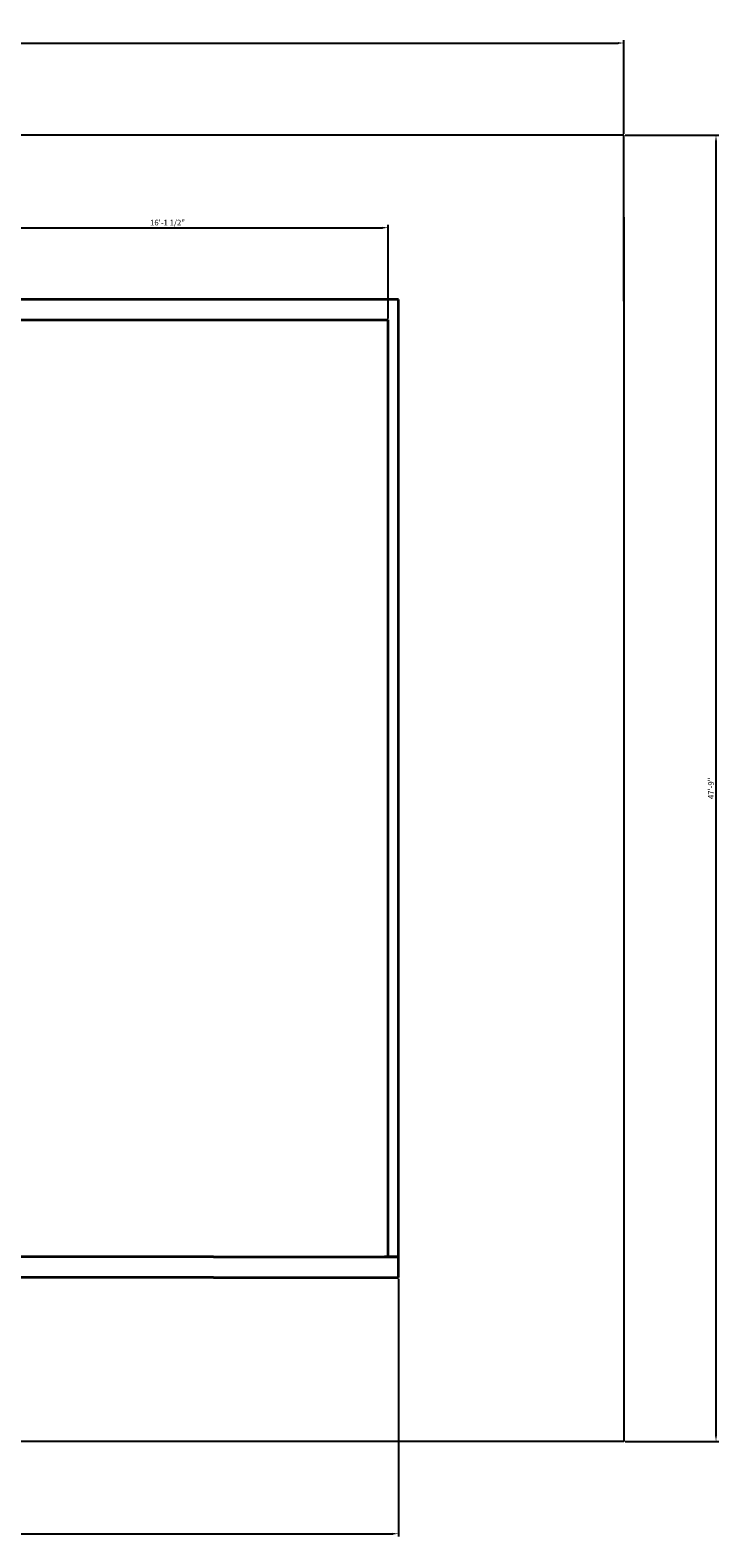
# Model space of a CAD drawing. Units: inches. Extents: x 250205121 to 250208111, y 89832590 to 89833271.
# Tile 14 of 14: x 250207809 to 250208111, y 89832598 to 89833259. Entities that reach past the tile are written whole.
import ezdxf

# ---------------------------------------------------------------- set-up
doc = ezdxf.new("R2010")
doc.units = ezdxf.units.IN
for name, color, linetype, lineweight in [('A-WALL', 7, 'Continuous', 35), ('C-PROP', 8, 'Continuous', 25), ('dimensions', 2, 'Continuous', 18)]:
    doc.layers.add(name, color=color, linetype=linetype, lineweight=lineweight)
doc.styles.get("Standard").update_dxf_attribs({"font": 'arial.ttf'})
doc.dimstyles.new('ISO-25', dxfattribs={"dimtxt": 2.5, "dimasz": 2.5, "dimexe": 1.25, "dimexo": 0.625, "dimtad": 1, "dimlunit": 4, "dimtxsty": 'Standard', "dimcen": 2.5, "dimadec": 0, "dimazin": 0, "dimtfac": 1, "dimtmove": 0, "dimatfit": 3, "dimfxl": 1, "dimarcsym": 0})

# ---------------------------------------------------------------- blocks, each defined once
blk = doc.blocks.new('*D66')
at = {"layer": 'Defpoints', "color": 0, "transparency": 16777216}
for p in [(250208069.71, 89833253.67), (250207267.21, 89833213.22), (250208069.71, 89833213.22)]:
    blk.add_point(p, dxfattribs=at)
at = {"layer": 'dimensions', "color": 0, "lineweight": -2, "transparency": 16777216}
for p, q in [((250207267.21, 89833213.84), (250207267.21, 89833254.92)), ((250208069.71, 89833213.84), (250208069.71, 89833254.92)), ((250207269.71, 89833253.67), (250208067.21, 89833253.67))]:
    blk.add_line(p, q, dxfattribs=at)
at = {"layer": 'dimensions', "color": 0, "transparency": 16777216}
for points in [[(250207269.71, 89833254.08), (250207269.71, 89833253.25), (250207267.21, 89833253.67)], [(250208067.21, 89833254.08), (250208067.21, 89833253.25), (250208069.71, 89833253.67)]]:
    blk.add_solid(points, dxfattribs=at)
at = {"layer": 'dimensions', "color": 0, "transparency": 16777216, "insert": (250207668.46, 89833255.58), "char_height": 2.5, "attachment_point": 5}
blk.add_mtext('66\'-10 1/2"', dxfattribs=at)
blk = doc.blocks.new('*D67')
at = {"layer": 'Defpoints', "color": 0, "transparency": 16777216}
for p in [(250208069.71, 89833213.22), (250208110.16, 89833213.22), (250208069.71, 89832640.22)]:
    blk.add_point(p, dxfattribs=at)
at = {"layer": 'dimensions', "color": 0, "lineweight": -2, "transparency": 16777216}
for p, q in [((250208070.33, 89833213.22), (250208111.41, 89833213.22)), ((250208110.16, 89832642.72), (250208110.16, 89833210.72)), ((250208070.33, 89832640.22), (250208111.41, 89832640.22))]:
    blk.add_line(p, q, dxfattribs=at)
at = {"layer": 'dimensions', "color": 0, "transparency": 16777216}
for points in [[(250208109.74, 89833210.72), (250208110.57, 89833210.72), (250208110.16, 89833213.22)], [(250208109.74, 89832642.72), (250208110.57, 89832642.72), (250208110.16, 89832640.22)]]:
    blk.add_solid(points, dxfattribs=at)
at = {"layer": 'dimensions', "color": 0, "transparency": 16777216, "insert": (250208108.26, 89832926.72), "char_height": 2.5, "attachment_point": 5, "rotation": 90}
blk.add_mtext('47\'-9"', dxfattribs=at)
blk = doc.blocks.new('*D70')
at = {"layer": 'Defpoints', "color": 0, "transparency": 16777216}
for p in [(250207339.21, 89832712.22), (250207970.87, 89832712.22), (250207970.87, 89832599.77)]:
    blk.add_point(p, dxfattribs=at)
at = {"layer": 'dimensions', "color": 0, "lineweight": -2, "transparency": 16777216}
for p, q in [((250207339.21, 89832711.59), (250207339.21, 89832598.52)), ((250207970.87, 89832711.59), (250207970.87, 89832598.52)), ((250207341.71, 89832599.77), (250207968.37, 89832599.77))]:
    blk.add_line(p, q, dxfattribs=at)
at = {"layer": 'dimensions', "color": 0, "transparency": 16777216}
for points in [[(250207341.71, 89832600.18), (250207341.71, 89832599.35), (250207339.21, 89832599.77)], [(250207968.37, 89832600.18), (250207968.37, 89832599.35), (250207970.87, 89832599.77)]]:
    blk.add_solid(points, dxfattribs=at)
at = {"layer": 'dimensions', "color": 0, "transparency": 16777216, "insert": (250207655.04, 89832601.68), "char_height": 2.5, "attachment_point": 5}
blk.add_mtext('52\'-7 1/2"', dxfattribs=at)
blk = doc.blocks.new('*D72')
at = {"layer": 'Defpoints', "color": 0, "transparency": 16777216}
for p in [(250207966.37, 89833172.67), (250207772.71, 89833132.22), (250207966.37, 89833132.22)]:
    blk.add_point(p, dxfattribs=at)
at = {"layer": 'dimensions', "color": 0, "lineweight": -2, "transparency": 16777216}
for p, q in [((250207772.71, 89833132.84), (250207772.71, 89833173.92)), ((250207775.21, 89833172.67), (250207963.87, 89833172.67)), ((250207966.37, 89833132.84), (250207966.37, 89833173.92))]:
    blk.add_line(p, q, dxfattribs=at)
at = {"layer": 'dimensions', "color": 0, "transparency": 16777216}
for points in [[(250207775.21, 89833173.08), (250207775.21, 89833172.25), (250207772.71, 89833172.67)], [(250207963.87, 89833173.08), (250207963.87, 89833172.25), (250207966.37, 89833172.67)]]:
    blk.add_solid(points, dxfattribs=at)
at = {"layer": 'dimensions', "color": 0, "transparency": 16777216, "insert": (250207869.54, 89833174.58), "char_height": 2.5, "attachment_point": 5}
blk.add_mtext('16\'-1 1/2"', dxfattribs=at)

msp = doc.modelspace()

# ---------------------------------------------------------------- linework, layer by layer
at = {"layer": 'A-WALL'}
for p, q in [((250207970.867, 89833141.217), (250207348.207, 89833141.217)), ((250207970.867, 89832712.217), (250207970.867, 89833141.217)), ((250207348.207, 89833132.217), (250207966.367, 89833132.217)), ((250207966.367, 89832721.217), (250207966.367, 89833132.217)), ((250207889.707, 89832721.217), (250207348.207, 89832721.217)), ((250207889.707, 89832721.217), (250207970.867, 89832721.217)), ((250207970.867, 89832721.217), (250207964.707, 89832721.217)), ((250207889.707, 89832712.217), (250207356.707, 89832712.217)), ((250207889.707, 89832712.217), (250207970.867, 89832712.217))]:
    msp.add_line(p, q, dxfattribs=at)
at = {"layer": 'C-PROP'}
for p, q in [((250208069.707, 89833213.217), (250207592.707, 89833213.217)), ((250208069.707, 89833177.217), (250208069.707, 89833213.217)), ((250208069.707, 89833140.463), (250208069.707, 89833177.217)), ((250208069.707, 89833177.217), (250208069.707, 89832640.217)), ((250208069.707, 89832976.217), (250208069.707, 89832976.217)), ((250208069.707, 89832640.217), (250207592.707, 89832640.217))]:
    msp.add_line(p, q, dxfattribs=at)

# ---------------------------------------------------------------- dimensions: what is measured, and where the dimension line sits
at = {"layer": 'dimensions'}
for base, p1, p2, picture, middle in [((250208069.707, 89833253.667), (250207267.207, 89833213.217), (250208069.707, 89833213.217), '*D66', (250207668.457, 89833255.585)), ((250207970.867, 89832599.767), (250207339.207, 89832712.217), (250207970.867, 89832712.217), '*D70', (250207655.037, 89832601.685))]:
    dim = msp.add_linear_dim(base=base, p1=p1, p2=p2, dimstyle='ISO-25', override={"dimdec": 1, "dimlfac": 1, "dimrnd": 0, "dimzin": 1, "dimdsep": 46, "dimlunit": 4, "dimfrac": 2}, dxfattribs=at)
    dim.commit()
    dim.dimension.update_dxf_attribs({"geometry": picture, "text_midpoint": middle})
for base, p1, p2, angle, picture, middle in [((250208110.157, 89833213.217), (250208069.707, 89832640.217), (250208069.707, 89833213.217), 90, '*D67', (250208108.256, 89832926.717)), ((250207966.367, 89833172.667), (250207772.707, 89833132.217), (250207966.367, 89833132.217), 0, '*D72', (250207869.537, 89833174.585))]:
    dim = msp.add_linear_dim(base=base, p1=p1, p2=p2, angle=angle, dimstyle='ISO-25', override={"dimdec": 1, "dimlfac": 1, "dimrnd": 0, "dimzin": 1, "dimdsep": 46, "dimlunit": 4, "dimfrac": 2}, dxfattribs=at)
    dim.commit()
    dim.dimension.update_dxf_attribs({"geometry": picture, "text_midpoint": middle})

doc.saveas('drawing.dxf')
